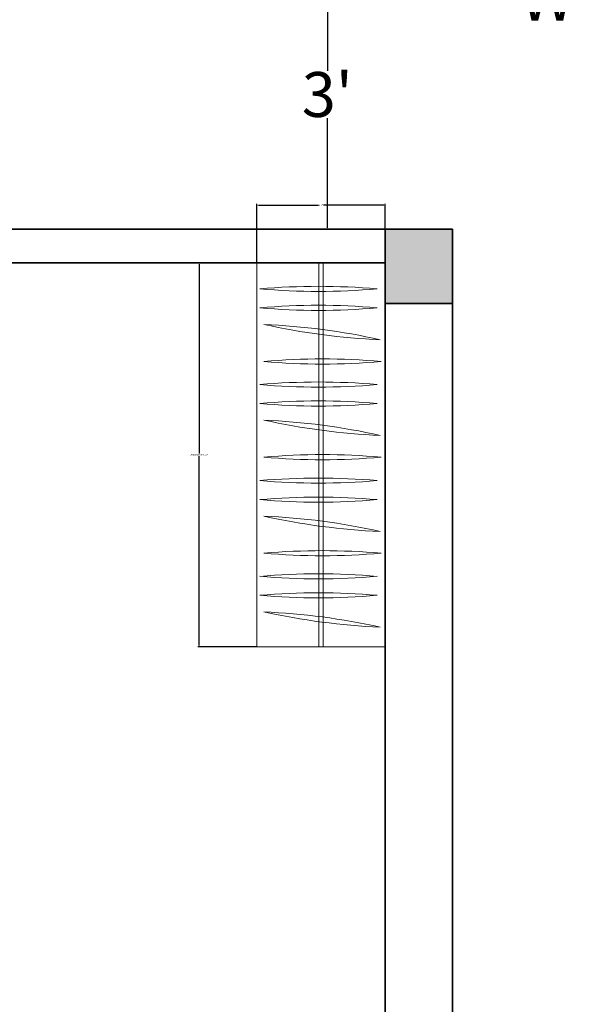
# Model space of a CAD drawing. Units: inches. Extents: x -36302355 to 648, y -221479757 to 75.
# Tile 28 of 37: x 265 to 341, y -271 to -139. Entities that reach past the tile are written whole.
import ezdxf

# ---------------------------------------------------------------- set-up
doc = ezdxf.new("R2010")
doc.units = ezdxf.units.IN
doc.header["$MEASUREMENT"] = 0
for name, color, linetype, lineweight in [('A-ANNO-DIMS', 2, 'Continuous', 18), ('A-ANNO-IDEN', 7, 'Continuous', 18), ('A-COLS', 7, 'Continuous', 35), ('A-COLS-PATT', 242, 'Continuous', 13), ('A-FURN', 8, 'Continuous', 13), ('A-WALL', 7, 'Continuous', 35)]:
    doc.layers.add(name, color=color, linetype=linetype, lineweight=lineweight)
doc.styles.get("Standard").update_dxf_attribs({"font": 'arial.ttf'})
doc.dimstyles.get("Standard").update_dxf_attribs({"dimtxt": 0.18, "dimasz": 0.18, "dimexe": 0.18, "dimexo": 0.0625, "dimgap": 0.09, "dimtad": 0, "dimtih": 1, "dimtoh": 1, "dimdec": 0, "dimzin": 0, "dimdsep": 46, "dimlunit": 3, "dimtxsty": 'Standard', "dimcen": 0.09, "dimadec": 0, "dimazin": 0, "dimtfac": 1, "dimtdec": 0, "dimtofl": 0, "dimtmove": 0, "dimatfit": 3, "dimfxl": 1, "dimtolj": 1, "dimtzin": 0, "dimarcsym": 0})

# ---------------------------------------------------------------- blocks, each defined once
blk = doc.blocks.new('*D1')
at = {"layer": 'A-ANNO-DIMS', "color": 0, "lineweight": -2, "transparency": 16777216}
for p, q in [((310.09, -131.02), (306.3, -131.02)), ((306.48, -131.2), (306.48, -145.86)), ((306.48, -166.84), (306.48, -152.17)), ((310.09, -167.02), (306.3, -167.02))]:
    blk.add_line(p, q, dxfattribs=at)
at = {"layer": 'A-ANNO-DIMS', "color": 0, "transparency": 16777216}
for points in [[(306.45, -131.2), (306.51, -131.2), (306.48, -131.02)], [(306.45, -166.84), (306.51, -166.84), (306.48, -167.02)]]:
    blk.add_solid(points, dxfattribs=at)
at = {"layer": 'Defpoints', "color": 0, "transparency": 16777216}
for p in [(310.15, -131.02), (306.48, -167.02), (310.15, -167.02)]:
    blk.add_point(p, dxfattribs=at)
at = {"layer": 'A-ANNO-DIMS', "color": 0, "transparency": 16777216, "insert": (306.48, -149.02), "char_height": 6, "attachment_point": 5}
blk.add_mtext("\\A1;3'", dxfattribs=at)
blk = doc.blocks.new('WARDROBE-HANGING')
for p, q in [((0, 0), (0, 53.32)), ((17.77, 53.32), (0, 53.32)), ((8.59, 0), (8.59, 53.32)), ((9.18, 0), (9.18, 53.32)), ((17.77, 0), (17.77, 53.32)), ((17.77, 0), (0, 0))]:
    blk.add_line(p, q)
for centre, start, end in [((8.53, -43.46), 85.0028, 94.9972), ((8.53, 142.85), 265.0028, 274.9972), ((8.53, -46.09), 85.0028, 94.9972), ((8.53, 140.22), 265.0028, 274.9972), ((21.18, 136.06), 257.508, 267.5023), ((-3.12, -48.66), 77.508, 87.5023), ((9.1, -53.54), 85.0028, 94.9972), ((9.1, 132.77), 265.0028, 274.9972), ((8.53, -56.74), 85.0028, 94.9972), ((8.53, 129.57), 265.0028, 274.9972), ((8.53, -59.37), 85.0028, 94.9972), ((8.53, 126.94), 265.0028, 274.9972), ((21.18, 122.78), 257.508, 267.5023), ((-3.12, -61.94), 77.508, 87.5023), ((9.1, -66.82), 85.0028, 94.9972), ((9.1, 119.49), 265.0028, 274.9972), ((8.53, -70.07), 85.0028, 94.9972), ((8.53, 116.24), 265.0028, 274.9972), ((8.53, -72.71), 85.0028, 94.9972), ((8.53, 113.6), 265.0028, 274.9972), ((-3.12, -75.27), 77.508, 87.5023), ((21.18, 109.44), 257.508, 267.5023), ((9.1, -80.15), 85.0028, 94.9972), ((9.1, 106.16), 265.0028, 274.9972), ((8.53, -83.36), 85.0028, 94.9972), ((8.53, 102.95), 265.0028, 274.9972), ((8.53, -85.99), 85.0028, 94.9972), ((8.53, 100.32), 265.0028, 274.9972), ((-3.12, -88.56), 77.508, 87.5023), ((21.18, 96.16), 257.508, 267.5023)]:
    blk.add_arc(centre, 93.51, start, end)
blk = doc.blocks.new('*D45')
at = {"layer": 'A-ANNO-DIMS', "color": 0, "lineweight": -2, "transparency": 16777216}
for p, q in [((297.02, -171.52), (289.19, -171.52)), ((289.37, -171.7), (289.37, -197.01)), ((289.37, -222.7), (289.37, -197.38)), ((297.02, -222.88), (289.19, -222.88))]:
    blk.add_line(p, q, dxfattribs=at)
at = {"layer": 'A-ANNO-DIMS', "color": 0, "transparency": 16777216}
for points in [[(289.34, -171.7), (289.4, -171.7), (289.37, -171.52)], [(289.34, -222.7), (289.4, -222.7), (289.37, -222.88)]]:
    blk.add_solid(points, dxfattribs=at)
at = {"layer": 'Defpoints', "color": 0, "transparency": 16777216}
for p in [(289.37, -171.52), (297.08, -171.52), (297.08, -222.88)]:
    blk.add_point(p, dxfattribs=at)
at = {"layer": 'A-ANNO-DIMS', "color": 0, "transparency": 16777216, "insert": (289.37, -197.2), "char_height": 0.18, "attachment_point": 5}
blk.add_mtext('\\A1;WARDROBE 4\'-3 1/2"', dxfattribs=at)
blk = doc.blocks.new('*D46')
at = {"layer": 'A-ANNO-DIMS', "color": 0, "lineweight": -2, "transparency": 16777216}
for p, q in [((297.08, -171.46), (297.08, -163.64)), ((297.26, -163.82), (305.32, -163.82)), ((314.02, -163.82), (305.96, -163.82)), ((314.2, -171.46), (314.2, -163.64))]:
    blk.add_line(p, q, dxfattribs=at)
at = {"layer": 'A-ANNO-DIMS', "color": 0, "transparency": 16777216}
for points in [[(297.26, -163.79), (297.26, -163.85), (297.08, -163.82)], [(314.02, -163.79), (314.02, -163.85), (314.2, -163.82)]]:
    blk.add_solid(points, dxfattribs=at)
at = {"layer": 'Defpoints', "color": 0, "transparency": 16777216}
for p in [(314.2, -163.82), (297.08, -171.52), (314.2, -171.52)]:
    blk.add_point(p, dxfattribs=at)
at = {"layer": 'A-ANNO-DIMS', "color": 0, "transparency": 16777216, "insert": (305.64, -163.82), "char_height": 0.18, "attachment_point": 5}
blk.add_mtext('\\A1;1\'-5"', dxfattribs=at)

msp = doc.modelspace()

# ---------------------------------------------------------------- hatches: boundary and pattern name
at = {"layer": 'A-COLS-PATT'}
h = msp.add_hatch(color=256, dxfattribs=at)
h.dxf.hatch_style = 1
h.paths.add_polyline_path([(145.2, 24.98), (145.2, 15.98), (154.2, 15.98), (154.2, 24.98)])
h.paths.add_polyline_path([(247.2, 15.98), (247.2, 24.98), (238.2, 24.98), (238.2, 15.98)])
h.paths.add_polyline_path([(387.64, 15.98), (395.7, 15.98), (395.7, 24.98), (387.64, 24.98)])
h.paths.add_polyline_path([(451.26, 24.98), (443.7, 24.98), (443.7, 15.98), (451.26, 15.98)])
h.paths.add_polyline_path([(596.2, 15.98), (605.2, 15.98), (605.2, 24.98), (596.2, 24.98)])
h.paths.add_polyline_path([(238.2, -122.02), (238.2, -131.02), (247.2, -131.02), (247.2, -122.02)])
h.paths.add_polyline_path([(395.7, -122.02), (387.46, -122.02), (387.46, -131.02), (395.7, -131.02)])
h.paths.add_polyline_path([(448.2, -131.02), (453.73, -131.02), (453.73, -122.02), (443.7, -122.02), (443.7, -131.02)])
h.paths.add_polyline_path([(596.2, -131.02), (605.2, -131.02), (605.2, -122.02), (596.2, -122.02)])
h.paths.add_polyline_path([(145.2, -176.97), (154.2, -176.97), (154.2, -167.02), (145.2, -167.02)])
h.paths.add_polyline_path([(314.2, -176.97), (323.2, -176.97), (323.2, -167.02), (314.2, -167.02)])
h.paths.add_polyline_path([(154.2, -314.02), (154.2, -309.52), (145.2, -309.52), (145.2, -314.02)])
h.paths.add_polyline_path([(314.2, -309.52), (314.2, -318.52), (323.2, -318.52), (323.2, -309.52)])
h.paths.add_polyline_path([(448.2, -277.02), (443.7, -277.02), (443.7, -286.02), (448.2, -286.02)])
h.paths.add_polyline_path([(283.2, -370.02), (274.2, -370.02), (274.2, -379.02), (283.2, -379.02), (283.2, -374.52)])
h.paths.add_polyline_path([(154.2, -370.02), (145.2, -370.02), (145.2, -379.02), (154.2, -379.02)])
h.paths.add_polyline_path([(443.2, -374.52), (443.2, -379.02), (452.2, -379.02), (452.2, -374.52)])
h.paths.add_polyline_path([(145.2, -580.02), (154.2, -580.02), (154.2, -571.02), (145.2, -571.02)])
h.paths.add_polyline_path([(274.2, -571.02), (274.2, -580.02), (283.2, -580.02), (283.2, -571.02)])
h.paths.add_polyline_path([(443.2, -580.02), (452.2, -580.02), (452.2, -571.02), (443.2, -571.02)])

# ---------------------------------------------------------------- linework, layer by layer
at = {"layer": 'A-COLS'}
msp.add_line((314.2, -176.97), (323.2, -176.97), dxfattribs=at)
at = {"layer": 'A-WALL'}
for p, q in [((145.2, -167.02), (323.2, -167.02)), ((314.2, -167.02), (314.2, -281.52)), ((323.2, -167.02), (323.2, -281.52)), ((154.2, -171.52), (314.2, -171.52))]:
    msp.add_line(p, q, dxfattribs=at)

# ---------------------------------------------------------------- block references
at = {"layer": 'A-FURN', "xscale": 0.963279288722585, "yscale": 0.963279288722585, "rotation": 8.537736463e-07}
msp.add_blockref('WARDROBE-HANGING', (297.08, -222.88), dxfattribs=at)

# ---------------------------------------------------------------- texts
at = {"layer": 'A-ANNO-IDEN', "insert": (332.27, -133.13), "char_height": 6, "attachment_point": 1}
msp.add_mtext_dynamic_manual_height_columns('W', width=2.1009, gutter_width=1, heights=[0], dxfattribs=at)

# ---------------------------------------------------------------- dimensions: what is measured, and where the dimension line sits
at = {"layer": 'A-ANNO-DIMS'}
for base, p1, p2, angle, override, picture, middle in [((306.48, -167.02), (310.15, -131.02), (310.15, -167.02), 90, {"dimtxt": 6, "dimclrd": 0, "dimclre": 0, "dimclrt": 0}, '*D1', (306.48, -149.02)), ((314.2, -163.82), (297.08, -171.52), (314.2, -171.52), 0, {"dimdec": 1, "dimlfac": 1, "dimrnd": 0, "dimzin": 1, "dimdsep": 46, "dimlunit": 4, "dimfrac": 2}, '*D46', (305.64, -163.82))]:
    dim = msp.add_linear_dim(base=base, p1=p1, p2=p2, angle=angle, dimstyle='Standard', override=override, dxfattribs=at)
    dim.commit()
    dim.dimension.update_dxf_attribs({"geometry": picture, "text_midpoint": middle})
dim = msp.add_linear_dim(base=(289.37, -171.52), p1=(297.08, -222.88), p2=(297.08, -171.52), angle=90, text='WARDROBE <>', dimstyle='Standard', override={"dimdec": 1, "dimlfac": 1, "dimrnd": 0, "dimzin": 1, "dimdsep": 46, "dimlunit": 4, "dimfrac": 2}, dxfattribs=at)
dim.commit()
dim.dimension.update_dxf_attribs({"geometry": '*D45', "text_midpoint": (289.37, -197.2)})

doc.saveas('drawing.dxf')
